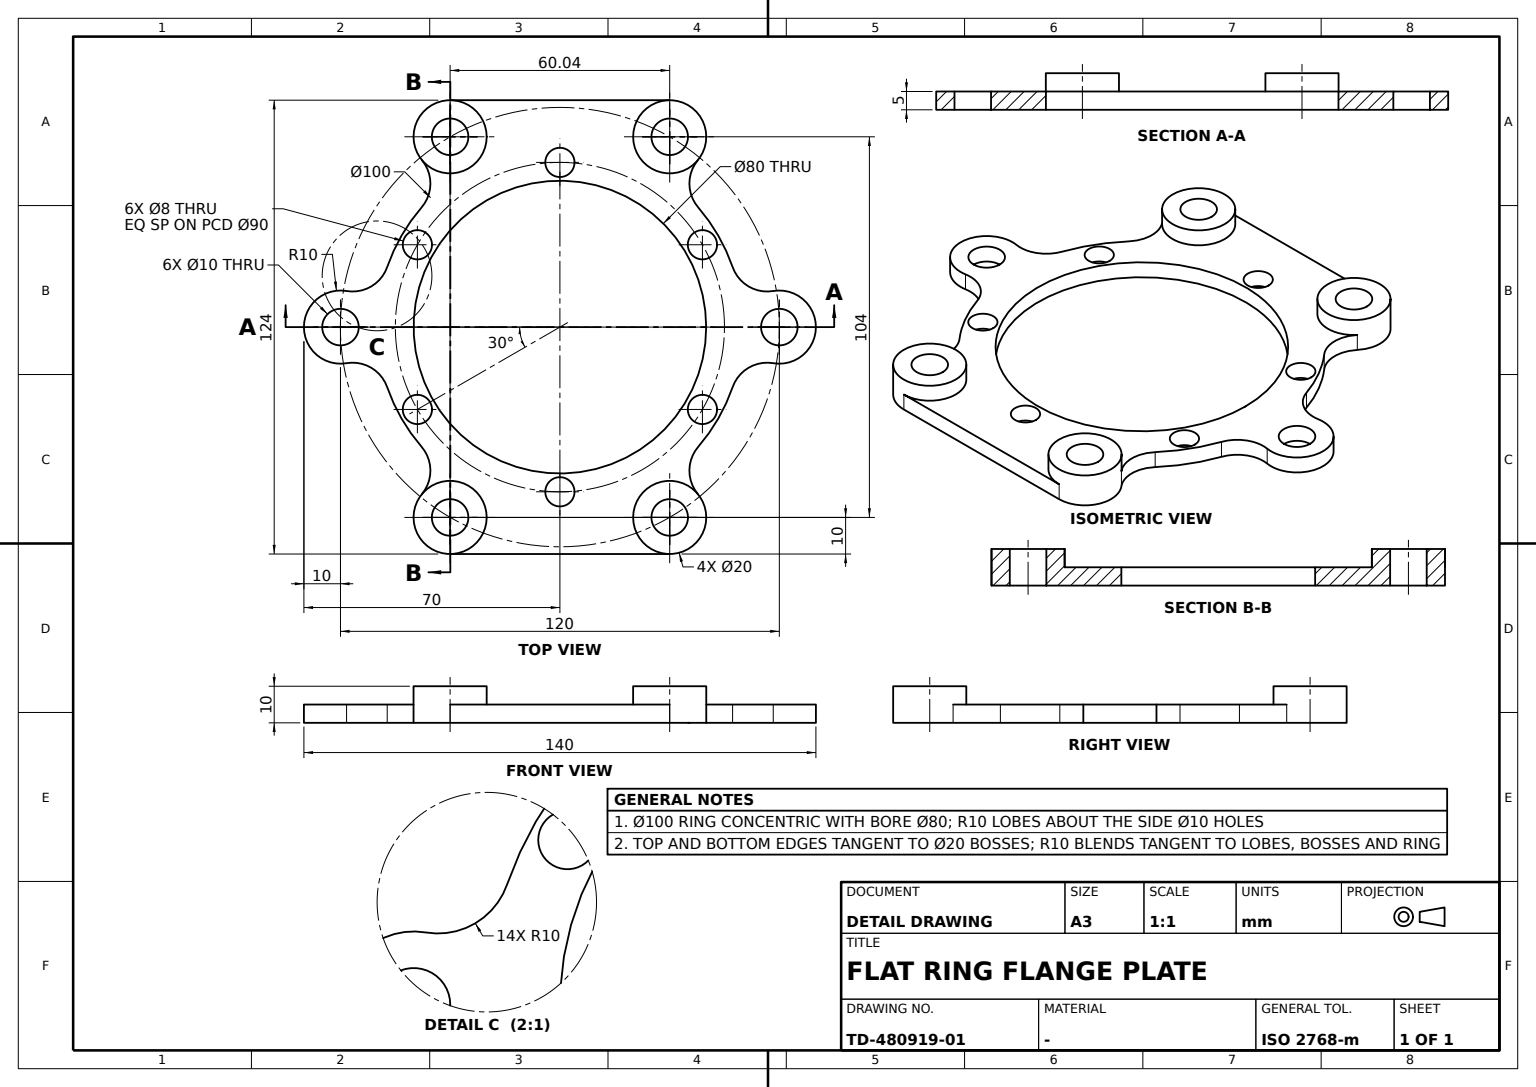
CATIA V5 part; units mm, degrees
sketch "Sketch1" plane through (0, 0, 0) normal (0, 0, 1) x (1, 0, 0)
  circle A0 centre (0, 0) radius 40
  circle A1 centre (0, 0) radius 60 construction
  arc A2 (-47.2222, -16.4336) -> (-37.8389, -32.6836) centre (0, 0) ccw
  line L0 (0, 0) -> (-53.9514, -93.4466) construction
  line L1 (0, 0) -> (53.9514, -93.4466) construction
  line L2 (0, 0) -> (-52.0877, 90.2185) construction
  line L3 (0, 0) -> (52.0877, 90.2185) construction
  arc A3 (30.0222, -62) -> (37.7144, -45.6102) centre (30.0222, -52) ccw
  point P0 (30.0222, -52)
  arc A4 (-37.7144, -45.6102) -> (-30.0222, -62) centre (-30.0222, -52) ccw
  point P1 (-30.0222, -52)
  arc A5 (37.7144, 45.6102) -> (30.0222, 62) centre (30.0222, 52) ccw
  point P2 (30.0222, 52)
  arc A6 (-30.0222, 62) -> (-37.7144, 45.6102) centre (-30.0222, 52) ccw
  point P3 (-30.0222, 52)
  arc A7 (58.3333, -9.8601) -> (58.3333, 9.8601) centre (60, 0) ccw
  point P4 (60, 0)
  arc A8 (-58.3333, 9.8601) -> (-58.3333, -9.8601) centre (-60, 0) ccw
  point P5 (-60, 0)
  arc A9 (37.7144, 45.6102) -> (37.8389, 32.6836) centre (45.4066, 39.2204) ccw
  arc A10 (47.2222, 16.4336) -> (58.3333, 9.8601) centre (56.6667, 19.7203) ccw
  point P6 (47.2222, 16.4336)
  arc A11 (58.3333, -9.8601) -> (47.2222, -16.4336) centre (56.6667, -19.7203) ccw
  arc A12 (37.7144, -45.6102) -> (37.8389, -32.6836) centre (45.4066, -39.2204) cw
  point P7 (37.8389, -32.6836)
  arc A13 (-37.7144, -45.6102) -> (-37.8389, -32.6836) centre (-45.4066, -39.2204) ccw
  arc A14 (-58.3333, -9.8601) -> (-47.2222, -16.4336) centre (-56.6667, -19.7203) cw
  arc A15 (-58.3333, 9.8601) -> (-47.2222, 16.4336) centre (-56.6667, 19.7203) ccw
  point P8 (-58.3333, 9.8601)
  arc A16 (-37.7144, 45.6102) -> (-37.8389, 32.6836) centre (-45.4066, 39.2204) cw
  point P9 (-37.8389, 32.6836)
  line L4 (30.0222, -62) -> (-30.0222, -62)
  line L5 (30.0222, 62) -> (-30.0222, 62)
  point P10 (-58.3333, 9.8601)
  arc A17 (-37.8389, 32.6836) -> (-47.2222, 16.4336) centre (0, 0) ccw
  arc A18 (47.2222, 16.4336) -> (37.8389, 32.6836) centre (0, 0) ccw
  arc A19 (37.8389, -32.6836) -> (47.2222, -16.4336) centre (0, 0) ccw
  circle A20 centre (30.0222, -52) radius 5
  point P11 (32.5222, -56.3301)
  circle A21 centre (-30.0222, -52) radius 5
  circle A22 centre (30.0222, 52) radius 5
  circle A23 centre (-30.0222, 52) radius 5
  circle A24 centre (60, 0) radius 5
  circle A25 centre (-60, 0) radius 5
  circle A26 centre (0, 0) radius 45 construction
  circle A27 centre (0, 45) radius 4
  point P12 (0, 45)
  point P13 (38.9711, 22.5)
  circle A28 centre (38.9711, 22.5) radius 4
  point P14 (38.9711, -22.5)
  circle A29 centre (38.9711, -22.5) radius 4
  point P15 (0, -45)
  circle A30 centre (0, -45) radius 4
  point P16 (-38.9711, -22.5)
  circle A31 centre (-38.9711, -22.5) radius 4
  point P17 (-38.9711, 22.5)
  circle A32 centre (-38.9711, 22.5) radius 4
  line L6 (38.9711, 22.5) -> (0, 0) construction
  line L7 (38.9711, -22.5) -> (0, 0) construction
  line L8 (0, -45) -> (0, 0) construction
  line L9 (-38.9711, -22.5) -> (0, 0) construction
  line L10 (0, 0) -> (-38.9711, 22.5) construction
  dimension "radius A0" = 40
  dimension "radius A1" = 60
  dimension "radius A2" = 50
  dimension "angle L1 y axis" = 30
  dimension "angle L0 y axis" = 30
  dimension "angle L3 y axis" = 30
  dimension "angle L2 y axis" = 30
  dimension "radius A3" = 10
  dimension "radius A4" = 10
  dimension "radius A5" = 10
  dimension "radius A6" = 10
  dimension "distance P2 x axis" = 52
  dimension "distance x axis P0" = 52
  dimension "distance P3 x axis" = 52
  dimension "distance P1 x axis" = 52
  dimension "radius A7" = 10
  dimension "radius A8" = 10
  dimension "radius A9" = 10
  dimension "radius A10" = 10
  dimension "radius A11" = 10
  dimension "radius A12" = 10
  dimension "radius A13" = 10
  dimension "radius A14" = 10
  dimension "radius A15" = 10
  dimension "radius A16" = 10
  dimension "radius A20" = 5
  dimension "radius A21" = 5
  dimension "radius A22" = 5
  dimension "radius A23" = 5
  dimension "radius A24" = 5
  dimension "radius A25" = 5
  dimension "radius A26" = 45
  dimension "radius A27" = 4
  dimension "radius A28" = 4
  dimension "radius A29" = 4
  dimension "radius A30" = 4
  dimension "radius A31" = 4
  dimension "radius A32" = 4
  dimension "angle L9 y axis" = 120
  constraint coincidence P0 L1
  constraint coincidence P1 L0
  constraint coincidence P2 L3
  constraint coincidence P3 L2
  constraint coincidence P4 A1
  constraint coincidence P4 x-axis
  constraint coincidence P5 A1
  constraint coincidence P5 x-axis
  constraint coincidence A2 P6
  constraint coincidence A2 P7
  constraint coincidence A8 P8
  constraint coincidence A2 P9
  constraint coincidence A15 P10
  constraint coincidence A2 A17
  constraint coincidence A2 A18
  constraint coincidence A2 A19
  constraint coincidence A20 P11
  constraint coincidence P11 L1
  constraint coincidence P12 A26
  constraint coincidence P12 y-axis
  constraint coincidence P13 A26
  constraint coincidence P14 A26
  constraint coincidence P15 A26
  constraint coincidence P16 A26
  constraint coincidence P17 A26
  constraint coincidence P8 P10
  constraint tangency A9 A5
  constraint tangency A9 A2
  constraint tangency A10 A2
  constraint tangency A10 A7
  constraint tangency A11 A7
  constraint tangency A11 A2
  constraint tangency A12 A3
  constraint tangency A12 A2
  constraint tangency A13 A4
  constraint tangency A13 A2
  constraint tangency A14 A8
  constraint tangency A14 A2
  constraint tangency A15 A8
  constraint tangency A15 A2
  constraint tangency A16 A6
  constraint tangency A16 A2
  constraint tangency L4 A4
  constraint tangency L4 A3
  constraint tangency L5 A6
  constraint tangency L5 A5
  constraint perpendicularity L6 L1
  constraint perpendicularity L7 L0
  constraint vertical L8 y-axis
  constraint parallelism L10 L7
extrude "Pad1" add sketch "Sketch1" against normal blind 5
sketch "Sketch2" plane through (0, 0, 0) normal (0, 0, 1) x (1, 0, 0)
  circle A0 centre (30.0222, 52) radius 5
  circle A1 centre (30.0222, 52) radius 10
  point P0 (30.0222, 52)
  arc A2 (37.7144, 45.6102) -> (30.0222, 62) centre (30.0222, 52) ccw construction
  circle A3 centre (-30.0222, 52) radius 5
  circle A4 centre (-30.0222, 52) radius 10
  point P1 (-30.0222, 52)
  arc A5 (-30.0222, 62) -> (-37.7144, 45.6102) centre (-30.0222, 52) ccw construction
  circle A6 centre (30.0222, -52) radius 5
  circle A7 centre (30.0222, -52) radius 10
  point P2 (30.0222, -52)
  arc A8 (30.0222, -62) -> (37.7144, -45.6102) centre (30.0222, -52) ccw construction
  circle A9 centre (-30.0222, -52) radius 5
  circle A10 centre (-30.0222, -52) radius 10
  point P3 (-30.0222, -52)
  arc A11 (-37.7144, -45.6102) -> (-30.0222, -62) centre (-30.0222, -52) ccw construction
  constraint concentricity P0 A0
  constraint concentricity P1 A3
  constraint concentricity P2 A6
  constraint concentricity P3 A9
  constraint coincidence A1 A2
  constraint coincidence A4 A5
  constraint coincidence A7 A8
  constraint coincidence A10 A11
extrude "Pad2" add sketch "Sketch2" along normal blind 5
